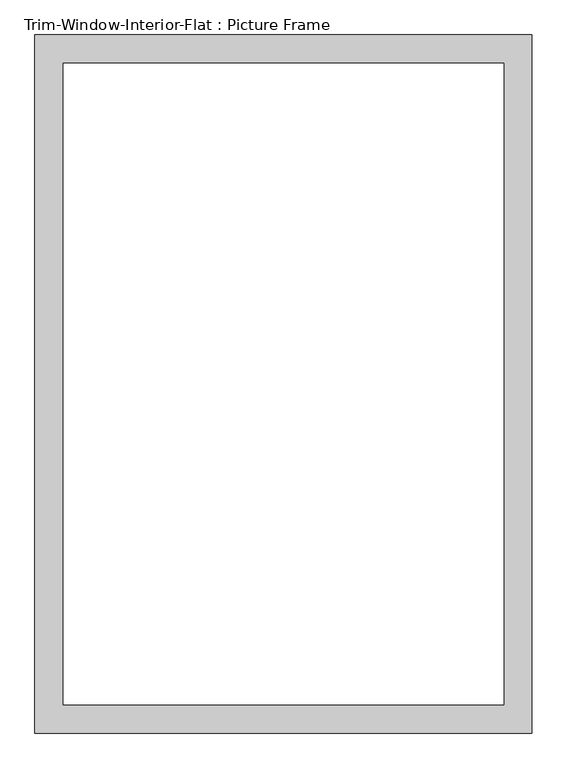
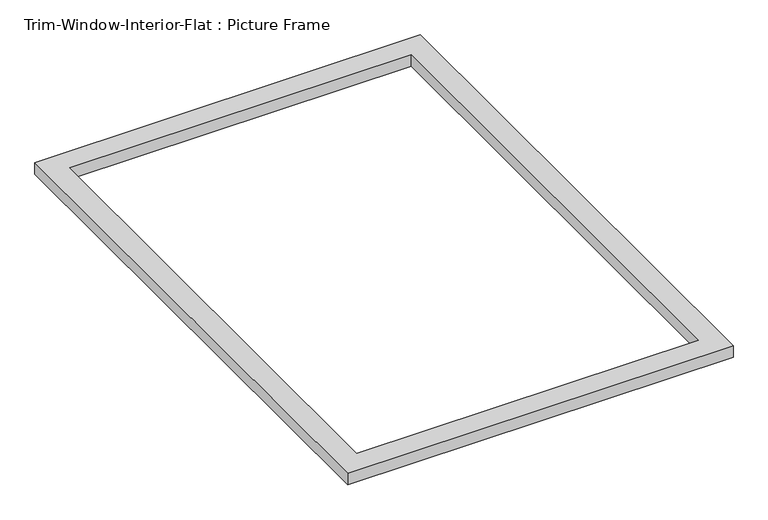
"""IFC4 building model written with IfcOpenShell, lengths in millimetres: proxy geometry, Trim-Window-Interior-Flat : Picture Frame."""

from ifc_helpers import new_model, si_unit, origin, origin_with_axes, place, context, project, spatial, polyline, outline, extrude, source, transform, mapped, element, save


def trim_window_interior_flat_picture_frame_db6fc9b7(model_context):
    return source(origin(), model_context, "Body", "SweptSolid", [
        extrude(outline(polyline([(501.65, 44.45), (501.65, -1365.25), (-501.65, -1365.25), (-501.65, 44.45), (501.65, 44.45)]), holes=[polyline([(444.5, -12.7), (-444.5, -12.7), (-444.5, -1308.1), (444.5, -1308.1), (444.5, -12.7)])]), origin_with_axes(), (0.0, 0.0, 1.0), 31.75),
    ])


if __name__ == "__main__":
    model = new_model("IFC4")
    model_context = context("Model", 3, world=origin())
    ifc_project = project(units=[si_unit("LENGTHUNIT", "METRE", prefix="MILLI")], contexts=[model_context])
    site = spatial("IfcSite", under=ifc_project)
    building = spatial("IfcBuilding", under=site)
    placement = place(None, origin())
    trim_window_interior_flat_picture_frame_shape = trim_window_interior_flat_picture_frame_db6fc9b7(model_context)
    element("IfcBuildingElementProxy", 1, Name="Trim-Window-Interior-Flat : Picture Frame", ObjectType="Trim-Window-Interior-Flat : Picture Frame", at=placement, inside=building, context=model_context, shape_type="MappedRepresentation", body=[
        mapped(trim_window_interior_flat_picture_frame_shape, transform((0.0, 0.0, 0.0), x_axis=(1.0, 0.0, 0.0), y_axis=(0.0, 1.0, 0.0), z_axis=(0.0, 0.0, 1.0))),
    ])
    save(model, "model.ifc")

# Revit data of these elements
# Type "Trim-Window-Interior-Flat : Picture Frame"
#   Trim Thickness_Picture Frame = 0' - 1 1/4"
#   Trim Width = 0' - 2 1/4"
#   Trim Thickness_with Sill = 0' - 0 3/4"
#   Sill Thickness = 0' - 1 1/4"
#   Opening Width [instance default] = 2' - 0"
#   Opening Height [instance default] = 3' - 0"
#   Default Elevation = 4' - 0"
#   Sill = no
#   Picture Frame = yes
#   Trim Material [instance default] = none
# Element 1 (IfcBuildingElementProxy, "Trim-Window-Interior-Flat : Picture Frame")
#   Opening Width = 3' - 0"
#   Opening Height = 4' - 4"
#   Trim Material = Wood - Stained
#   Materials on its faces: "Wood - Stained"
# Materials
#   "Wood - Stained": class "Wood", colour RGB 224 178 126, transparency 0, Cost = 0
